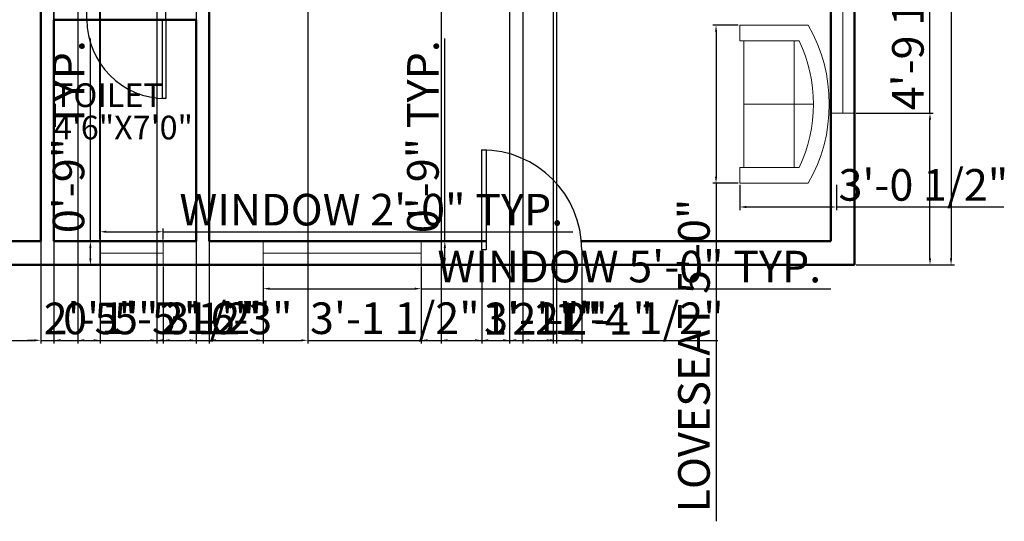
# Model space of a CAD drawing. Units: inches. Extents: x 2744 to 3775, y 2156 to 2963.
# Tile 2 of 4: x 3167 to 3541, y 2156 to 2346. Entities that reach past the tile are written whole.
import ezdxf

# ---------------------------------------------------------------- set-up
doc = ezdxf.new("R2010")
doc.units = ezdxf.units.IN
for name, color, linetype, lineweight in [('A-ANNO-DIMS', 2, 'Continuous', 18), ('A-AREA-IDEN', 7, 'Continuous', 25), ('A-DOOR', 3, 'Continuous', 25), ('A-FURN', 8, 'Continuous', 18), ('A-GLAZ', 4, 'Continuous', 18), ('A-WALL', 7, 'Continuous', 50)]:
    doc.layers.add(name, color=color, linetype=linetype, lineweight=lineweight)
doc.styles.get("Standard").update_dxf_attribs({"font": 'arial.ttf'})
doc.dimstyles.new('ISO-25', dxfattribs={"dimtxt": 12, "dimasz": 2.5, "dimexe": 1.25, "dimexo": 0.625, "dimtad": 1, "dimdec": 1, "dimlunit": 4, "dimtxsty": 'Standard', "dimcen": 2.5, "dimadec": 0, "dimazin": 0, "dimtfac": 1, "dimtdec": 1, "dimtmove": 0, "dimatfit": 3, "dimfxl": 1, "dimarcsym": 0})

# ---------------------------------------------------------------- blocks, each defined once
blk = doc.blocks.new('*U2')
for p, q in [((0, 0), (0, -6)), ((40, 0), (40, -6))]:
    blk.add_line(p, q)
blk.add_lwpolyline([(0, 0), (0, 40), (1.75, 40), (1.75, 0)], close=True)
blk.add_arc((0, 0), 40, 0, 90)
blk = doc.blocks.new('Sofa - Roundback Loveseat 5 ft.')
for p, q in [((0, -32.44198), (0, -5.99998)), ((-24, -33.99998), (-24, -11.46958)), ((-23.9998, -13.38178), (23.99986, -13.38178)), ((24.00004, -33.99998), (24.00004, -11.46958)), ((-24, -32.44198), (24.00004, -32.44198))]:
    blk.add_line(p, q)
for points in [[(-24, -33.99998), (-30, -33.99998), (-30, -7.99998)], [(30.00004, -7.99998), (30.00004, -33.99998), (24.00004, -33.99998)]]:
    blk.add_lwpolyline(points)
for centre, radius, start, end in [((0, -60.24998), 60.24998, 60.13715, 119.8628), ((0, -61.38438), 55.38444, 64.32083, 115.6792)]:
    blk.add_arc(centre, radius, start, end)
blk = doc.blocks.new('*D15')
at = {"layer": 'A-ANNO-DIMS', "color": 0, "lineweight": -2, "transparency": 16777216}
for p, q in [((3484.55, 2757.1), (3521.77, 2757.1)), ((3520.52, 2754.6), (3520.52, 2255.6)), ((3484.55, 2253.1), (3521.77, 2253.1))]:
    blk.add_line(p, q, dxfattribs=at)
at = {"layer": 'A-ANNO-DIMS', "color": 0, "transparency": 16777216}
for points in [[(3520.11, 2754.6), (3520.94, 2754.6), (3520.52, 2757.1)], [(3520.11, 2255.6), (3520.94, 2255.6), (3520.52, 2253.1)]]:
    blk.add_solid(points, dxfattribs=at)
at = {"layer": 'Defpoints', "color": 0, "transparency": 16777216}
for p in [(3483.92, 2757.1), (3483.92, 2253.1), (3520.52, 2253.1)]:
    blk.add_point(p, dxfattribs=at)
at = {"layer": 'A-ANNO-DIMS', "color": 0, "transparency": 16777216, "insert": (3513.88, 2505.1), "char_height": 12, "attachment_point": 5, "rotation": 90}
blk.add_mtext("42'", dxfattribs=at)
blk = doc.blocks.new('WIN-60IN')
blk.add_line((0, 4.5), (60, 4.5))
blk.add_lwpolyline([(0, 9), (60, 9), (60, 0), (0, 0)], close=True)
blk = doc.blocks.new('WIN-24IN')
blk.add_line((0, 4.5), (24, 4.5))
blk.add_lwpolyline([(0, 9), (24, 9), (24, 0), (0, 0)], close=True)
blk = doc.blocks.new('*D18')
at = {"layer": 'A-ANNO-DIMS', "color": 0, "lineweight": -2, "transparency": 16777216}
for p, q in [((3259.32, 2252.48), (3259.32, 2242.85)), ((3319.32, 2252.48), (3319.32, 2242.85)), ((3261.82, 2244.1), (3316.82, 2244.1)), ((3319.32, 2244.1), (3474.92, 2244.1))]:
    blk.add_line(p, q, dxfattribs=at)
at = {"layer": 'A-ANNO-DIMS', "color": 0, "transparency": 16777216}
for points in [[(3261.82, 2244.52), (3261.82, 2243.69), (3259.32, 2244.1)], [(3316.82, 2244.52), (3316.82, 2243.69), (3319.32, 2244.1)]]:
    blk.add_solid(points, dxfattribs=at)
at = {"layer": 'Defpoints', "color": 0, "transparency": 16777216}
for p in [(3259.32, 2253.1), (3319.32, 2253.1), (3319.32, 2244.1)]:
    blk.add_point(p, dxfattribs=at)
at = {"layer": 'A-ANNO-DIMS', "color": 0, "transparency": 16777216, "insert": (3398.37, 2250.94), "char_height": 12, "attachment_point": 5}
blk.add_mtext('WINDOW 5\'-0" TYP.', dxfattribs=at)
blk = doc.blocks.new('*D19')
at = {"layer": 'A-ANNO-DIMS', "color": 0, "lineweight": -2, "transparency": 16777216}
for p, q in [((3328.32, 2262.1), (3328.32, 2339)), ((3319.95, 2262.1), (3329.57, 2262.1)), ((3328.32, 2255.6), (3328.32, 2259.6)), ((3319.95, 2253.1), (3329.57, 2253.1))]:
    blk.add_line(p, q, dxfattribs=at)
at = {"layer": 'A-ANNO-DIMS', "color": 0, "transparency": 16777216}
for points in [[(3327.91, 2259.6), (3328.74, 2259.6), (3328.32, 2262.1)], [(3327.91, 2255.6), (3328.74, 2255.6), (3328.32, 2253.1)]]:
    blk.add_solid(points, dxfattribs=at)
at = {"layer": 'Defpoints', "color": 0, "transparency": 16777216}
for p in [(3319.32, 2262.1), (3328.32, 2262.1), (3319.32, 2253.1)]:
    blk.add_point(p, dxfattribs=at)
at = {"layer": 'A-ANNO-DIMS', "color": 0, "transparency": 16777216, "insert": (3321.57, 2301.8), "char_height": 12, "attachment_point": 5, "rotation": 90}
blk.add_mtext('0\'-9" TYP.', dxfattribs=at)
blk = doc.blocks.new('*D20')
at = {"layer": 'A-ANNO-DIMS', "color": 0, "lineweight": -2, "transparency": 16777216}
for p, q in [((3197.36, 2262.73), (3197.36, 2266.95)), ((3199.86, 2265.7), (3218.86, 2265.7)), ((3221.36, 2262.73), (3221.36, 2266.95)), ((3221.36, 2265.7), (3376.96, 2265.7))]:
    blk.add_line(p, q, dxfattribs=at)
at = {"layer": 'A-ANNO-DIMS', "color": 0, "transparency": 16777216}
for points in [[(3199.86, 2266.12), (3199.86, 2265.29), (3197.36, 2265.7)], [(3218.86, 2266.12), (3218.86, 2265.29), (3221.36, 2265.7)]]:
    blk.add_solid(points, dxfattribs=at)
at = {"layer": 'Defpoints', "color": 0, "transparency": 16777216}
for p in [(3221.36, 2265.7), (3197.36, 2262.1), (3221.36, 2262.1)]:
    blk.add_point(p, dxfattribs=at)
at = {"layer": 'A-ANNO-DIMS', "color": 0, "transparency": 16777216, "insert": (3300.41, 2272.54), "char_height": 12, "attachment_point": 5}
blk.add_mtext('WINDOW 2\'-0" TYP.', dxfattribs=at)
blk = doc.blocks.new('*D21')
at = {"layer": 'A-ANNO-DIMS', "color": 0, "lineweight": -2, "transparency": 16777216}
for p, q in [((3193.76, 2262.1), (3193.76, 2339)), ((3196.74, 2262.1), (3192.51, 2262.1)), ((3193.76, 2255.6), (3193.76, 2259.6)), ((3196.74, 2253.1), (3192.51, 2253.1))]:
    blk.add_line(p, q, dxfattribs=at)
at = {"layer": 'A-ANNO-DIMS', "color": 0, "transparency": 16777216}
for points in [[(3193.35, 2259.6), (3194.18, 2259.6), (3193.76, 2262.1)], [(3193.35, 2255.6), (3194.18, 2255.6), (3193.76, 2253.1)]]:
    blk.add_solid(points, dxfattribs=at)
at = {"layer": 'Defpoints', "color": 0, "transparency": 16777216}
for p in [(3193.76, 2262.1), (3197.36, 2262.1), (3197.36, 2253.1)]:
    blk.add_point(p, dxfattribs=at)
at = {"layer": 'A-ANNO-DIMS', "color": 0, "transparency": 16777216, "insert": (3187.01, 2301.8), "char_height": 12, "attachment_point": 5, "rotation": 90}
blk.add_mtext('0\'-9" TYP.', dxfattribs=at)
blk = doc.blocks.new('*D28')
at = {"layer": 'A-ANNO-DIMS', "color": 0, "lineweight": -2, "transparency": 16777216}
for p, q in [((3439.68, 2344.11), (3430.05, 2344.11)), ((3431.3, 2341.61), (3431.3, 2286.61)), ((3439.68, 2284.11), (3430.05, 2284.11)), ((3431.3, 2284.11), (3431.3, 2155.82))]:
    blk.add_line(p, q, dxfattribs=at)
at = {"layer": 'A-ANNO-DIMS', "color": 0, "transparency": 16777216}
for points in [[(3430.89, 2341.61), (3431.72, 2341.61), (3431.3, 2344.11)], [(3430.89, 2286.61), (3431.72, 2286.61), (3431.3, 2284.11)]]:
    blk.add_solid(points, dxfattribs=at)
at = {"layer": 'Defpoints', "color": 0, "transparency": 16777216}
for p in [(3440.3, 2344.11), (3431.3, 2284.11), (3440.3, 2284.11)]:
    blk.add_point(p, dxfattribs=at)
at = {"layer": 'A-ANNO-DIMS', "color": 0, "transparency": 16777216, "insert": (3424.47, 2218.72), "char_height": 12, "attachment_point": 5, "rotation": 90}
blk.add_mtext('LOVESEAT 5\'-0"', dxfattribs=at)
blk = doc.blocks.new('*D29')
at = {"layer": 'A-ANNO-DIMS', "color": 0, "lineweight": -2, "transparency": 16777216}
for p, q in [((3440.3, 2283.48), (3440.3, 2273.86)), ((3476.97, 2283.48), (3476.97, 2273.86)), ((3442.8, 2275.11), (3474.47, 2275.11)), ((3476.97, 2275.11), (3540.57, 2275.11))]:
    blk.add_line(p, q, dxfattribs=at)
at = {"layer": 'A-ANNO-DIMS', "color": 0, "transparency": 16777216}
for points in [[(3442.8, 2275.52), (3442.8, 2274.69), (3440.3, 2275.11)], [(3474.47, 2275.52), (3474.47, 2274.69), (3476.97, 2275.11)]]:
    blk.add_solid(points, dxfattribs=at)
at = {"layer": 'Defpoints', "color": 0, "transparency": 16777216}
for p in [(3440.3, 2284.11), (3476.97, 2284.11), (3476.97, 2275.11)]:
    blk.add_point(p, dxfattribs=at)
at = {"layer": 'A-ANNO-DIMS', "color": 0, "transparency": 16777216, "insert": (3510.02, 2281.94), "char_height": 12, "attachment_point": 5}
blk.add_mtext('3\'-0 1/2"', dxfattribs=at)
blk = doc.blocks.new('*D34')
at = {"layer": 'A-ANNO-DIMS', "color": 0, "lineweight": -2, "transparency": 16777216}
for p, q in [((3145.86, 2747.48), (3145.86, 2223.25)), ((3174.92, 2747.48), (3174.92, 2223.25)), ((3148.36, 2224.5), (3172.42, 2224.5)), ((3174.92, 2224.5), (3210.78, 2224.5))]:
    blk.add_line(p, q, dxfattribs=at)
at = {"layer": 'A-ANNO-DIMS', "color": 0, "transparency": 16777216}
for points in [[(3148.36, 2224.92), (3148.36, 2224.09), (3145.86, 2224.5)], [(3172.42, 2224.92), (3172.42, 2224.09), (3174.92, 2224.5)]]:
    blk.add_solid(points, dxfattribs=at)
at = {"layer": 'Defpoints', "color": 0, "transparency": 16777216}
for p in [(3145.86, 2748.1), (3174.92, 2748.1), (3174.92, 2224.5)]:
    blk.add_point(p, dxfattribs=at)
at = {"layer": 'A-ANNO-DIMS', "color": 0, "transparency": 16777216, "insert": (3194.1, 2231.26), "char_height": 12, "attachment_point": 5}
blk.add_mtext('2\'-5"', dxfattribs=at)
blk = doc.blocks.new('*D35')
at = {"layer": 'A-ANNO-DIMS', "color": 0, "lineweight": -2, "transparency": 16777216}
for p, q in [((3179.92, 2747.48), (3179.92, 2223.25)), ((3197.52, 2747.48), (3197.52, 2223.25)), ((3182.42, 2224.5), (3195.02, 2224.5)), ((3197.52, 2224.5), (3260.01, 2224.5))]:
    blk.add_line(p, q, dxfattribs=at)
at = {"layer": 'A-ANNO-DIMS', "color": 0, "transparency": 16777216}
for points in [[(3182.42, 2224.92), (3182.42, 2224.09), (3179.92, 2224.5)], [(3195.02, 2224.92), (3195.02, 2224.09), (3197.52, 2224.5)]]:
    blk.add_solid(points, dxfattribs=at)
at = {"layer": 'Defpoints', "color": 0, "transparency": 16777216}
for p in [(3179.92, 2748.1), (3197.52, 2748.1), (3197.52, 2224.5)]:
    blk.add_point(p, dxfattribs=at)
at = {"layer": 'A-ANNO-DIMS', "color": 0, "transparency": 16777216, "insert": (3230.02, 2231.33), "char_height": 12, "attachment_point": 5}
blk.add_mtext('1\'-5 1/2"', dxfattribs=at)
blk = doc.blocks.new('*D36')
at = {"layer": 'A-ANNO-DIMS', "color": 0, "lineweight": -2, "transparency": 16777216}
for p, q in [((3326.88, 2747.48), (3326.88, 2223.25)), ((3352.92, 2747.48), (3352.92, 2223.25)), ((3329.38, 2224.5), (3350.42, 2224.5)), ((3352.92, 2224.5), (3388.78, 2224.5))]:
    blk.add_line(p, q, dxfattribs=at)
at = {"layer": 'A-ANNO-DIMS', "color": 0, "transparency": 16777216}
for points in [[(3329.38, 2224.92), (3329.38, 2224.09), (3326.88, 2224.5)], [(3350.42, 2224.92), (3350.42, 2224.09), (3352.92, 2224.5)]]:
    blk.add_solid(points, dxfattribs=at)
at = {"layer": 'Defpoints', "color": 0, "transparency": 16777216}
for p in [(3326.88, 2748.1), (3352.92, 2748.1), (3352.92, 2224.5)]:
    blk.add_point(p, dxfattribs=at)
at = {"layer": 'A-ANNO-DIMS', "color": 0, "transparency": 16777216, "insert": (3372.1, 2231.15), "char_height": 12, "attachment_point": 5}
blk.add_mtext('2\'-2"', dxfattribs=at)
blk = doc.blocks.new('*D37')
at = {"layer": 'A-ANNO-DIMS', "color": 0, "lineweight": -2, "transparency": 16777216}
for p, q in [((3357.92, 2747.48), (3357.92, 2223.25)), ((3370.78, 2747.48), (3370.78, 2223.25)), ((3360.42, 2224.5), (3368.28, 2224.5)), ((3370.78, 2224.5), (3405.3, 2224.5))]:
    blk.add_line(p, q, dxfattribs=at)
at = {"layer": 'A-ANNO-DIMS', "color": 0, "transparency": 16777216}
for points in [[(3360.42, 2224.92), (3360.42, 2224.09), (3357.92, 2224.5)], [(3368.28, 2224.92), (3368.28, 2224.09), (3370.78, 2224.5)]]:
    blk.add_solid(points, dxfattribs=at)
at = {"layer": 'Defpoints', "color": 0, "transparency": 16777216}
for p in [(3357.92, 2748.1), (3370.78, 2748.1), (3370.78, 2224.5)]:
    blk.add_point(p, dxfattribs=at)
at = {"layer": 'A-ANNO-DIMS', "color": 0, "transparency": 16777216, "insert": (3389.29, 2231.15), "char_height": 12, "attachment_point": 5}
blk.add_mtext('1\'-1"', dxfattribs=at)
blk = doc.blocks.new('*D39')
at = {"layer": 'A-ANNO-DIMS', "color": 0, "lineweight": -2, "transparency": 16777216}
for p, q in [((3179.92, 2262.73), (3179.92, 2786.95)), ((3182.42, 2785.7), (3194.86, 2785.7)), ((3197.36, 2262.73), (3197.36, 2786.95)), ((3197.36, 2785.7), (3259.85, 2785.7))]:
    blk.add_line(p, q, dxfattribs=at)
at = {"layer": 'A-ANNO-DIMS', "color": 0, "transparency": 16777216}
for points in [[(3182.42, 2786.12), (3182.42, 2785.29), (3179.92, 2785.7)], [(3194.86, 2786.12), (3194.86, 2785.29), (3197.36, 2785.7)]]:
    blk.add_solid(points, dxfattribs=at)
at = {"layer": 'Defpoints', "color": 0, "transparency": 16777216}
for p in [(3197.36, 2785.7), (3179.92, 2262.1), (3197.36, 2262.1)]:
    blk.add_point(p, dxfattribs=at)
at = {"layer": 'A-ANNO-DIMS', "color": 0, "transparency": 16777216, "insert": (3229.85, 2792.53), "char_height": 12, "attachment_point": 5}
blk.add_mtext('1\'-5 1/2"', dxfattribs=at)
blk = doc.blocks.new('*D40')
at = {"layer": 'A-ANNO-DIMS', "color": 0, "lineweight": -2, "transparency": 16777216}
for p, q in [((3221.36, 2252.48), (3221.36, 2223.25)), ((3259.32, 2252.48), (3259.32, 2223.25)), ((3223.86, 2224.5), (3256.82, 2224.5))]:
    blk.add_line(p, q, dxfattribs=at)
at = {"layer": 'A-ANNO-DIMS', "color": 0, "transparency": 16777216}
for points in [[(3223.86, 2224.92), (3223.86, 2224.09), (3221.36, 2224.5)], [(3256.82, 2224.92), (3256.82, 2224.09), (3259.32, 2224.5)]]:
    blk.add_solid(points, dxfattribs=at)
at = {"layer": 'Defpoints', "color": 0, "transparency": 16777216}
for p in [(3221.36, 2253.1), (3259.32, 2253.1), (3259.32, 2224.5)]:
    blk.add_point(p, dxfattribs=at)
at = {"layer": 'A-ANNO-DIMS', "color": 0, "transparency": 16777216, "insert": (3240.34, 2231.26), "char_height": 12, "attachment_point": 5}
blk.add_mtext('3\'-2"', dxfattribs=at)
blk = doc.blocks.new('*D41')
at = {"layer": 'A-ANNO-DIMS', "color": 0, "lineweight": -2, "transparency": 16777216}
for p, q in [((3319.32, 2252.48), (3319.32, 2223.25)), ((3342.33, 2252.48), (3342.33, 2223.25)), ((3321.82, 2224.5), (3339.83, 2224.5)), ((3342.33, 2224.5), (3386.18, 2224.5))]:
    blk.add_line(p, q, dxfattribs=at)
at = {"layer": 'A-ANNO-DIMS', "color": 0, "transparency": 16777216}
for points in [[(3321.82, 2224.92), (3321.82, 2224.09), (3319.32, 2224.5)], [(3339.83, 2224.92), (3339.83, 2224.09), (3342.33, 2224.5)]]:
    blk.add_solid(points, dxfattribs=at)
at = {"layer": 'Defpoints', "color": 0, "transparency": 16777216}
for p in [(3319.32, 2253.1), (3342.33, 2253.1), (3342.33, 2224.5)]:
    blk.add_point(p, dxfattribs=at)
at = {"layer": 'A-ANNO-DIMS', "color": 0, "transparency": 16777216, "insert": (3365.5, 2231.15), "char_height": 12, "attachment_point": 5}
blk.add_mtext('1\'-11"', dxfattribs=at)
blk = doc.blocks.new('*D42')
at = {"layer": 'A-ANNO-DIMS', "color": 0, "lineweight": -2, "transparency": 16777216}
for p, q in [((3342.33, 2252.48), (3342.33, 2223.25)), ((3380.33, 2252.48), (3380.33, 2223.25)), ((3344.83, 2224.5), (3377.83, 2224.5))]:
    blk.add_line(p, q, dxfattribs=at)
at = {"layer": 'A-ANNO-DIMS', "color": 0, "transparency": 16777216}
for points in [[(3344.83, 2224.92), (3344.83, 2224.09), (3342.33, 2224.5)], [(3377.83, 2224.92), (3377.83, 2224.09), (3380.33, 2224.5)]]:
    blk.add_solid(points, dxfattribs=at)
at = {"layer": 'Defpoints', "color": 0, "transparency": 16777216}
for p in [(3342.33, 2253.1), (3380.33, 2253.1), (3380.33, 2224.5)]:
    blk.add_point(p, dxfattribs=at)
at = {"layer": 'A-ANNO-DIMS', "color": 0, "transparency": 16777216, "insert": (3361.33, 2231.26), "char_height": 12, "attachment_point": 5}
blk.add_mtext('3\'-2"', dxfattribs=at)
blk = doc.blocks.new('*D43')
at = {"layer": 'A-ANNO-DIMS', "color": 0, "lineweight": -2, "transparency": 16777216}
for p, q in [((3512.52, 2310.69), (3512.52, 2374.78)), ((3484.55, 2310.69), (3513.77, 2310.69)), ((3512.52, 2255.6), (3512.52, 2308.19)), ((3484.55, 2253.1), (3513.77, 2253.1))]:
    blk.add_line(p, q, dxfattribs=at)
at = {"layer": 'A-ANNO-DIMS', "color": 0, "transparency": 16777216}
for points in [[(3512.11, 2308.19), (3512.94, 2308.19), (3512.52, 2310.69)], [(3512.11, 2255.6), (3512.94, 2255.6), (3512.52, 2253.1)]]:
    blk.add_solid(points, dxfattribs=at)
at = {"layer": 'Defpoints', "color": 0, "transparency": 16777216}
for p in [(3483.92, 2310.69), (3512.52, 2310.69), (3483.92, 2253.1)]:
    blk.add_point(p, dxfattribs=at)
at = {"layer": 'A-ANNO-DIMS', "color": 0, "transparency": 16777216, "insert": (3505.69, 2343.99), "char_height": 12, "attachment_point": 5, "rotation": 90}
blk.add_mtext('4\'-9 1/2"', dxfattribs=at)
blk = doc.blocks.new('*D45')
at = {"layer": 'A-ANNO-DIMS', "color": 0, "lineweight": -2, "transparency": 16777216}
for p, q in [((3188.98, 2574.48), (3188.98, 2223.25)), ((3218.98, 2574.48), (3218.98, 2223.25)), ((3191.48, 2224.5), (3216.48, 2224.5)), ((3218.98, 2224.5), (3254.83, 2224.5))]:
    blk.add_line(p, q, dxfattribs=at)
at = {"layer": 'A-ANNO-DIMS', "color": 0, "transparency": 16777216}
for points in [[(3191.48, 2224.92), (3191.48, 2224.09), (3188.98, 2224.5)], [(3216.48, 2224.92), (3216.48, 2224.09), (3218.98, 2224.5)]]:
    blk.add_solid(points, dxfattribs=at)
at = {"layer": 'Defpoints', "color": 0, "transparency": 16777216}
for p in [(3188.98, 2575.1), (3218.98, 2575.1), (3218.98, 2224.5)]:
    blk.add_point(p, dxfattribs=at)
at = {"layer": 'A-ANNO-DIMS', "color": 0, "transparency": 16777216, "insert": (3238.16, 2231.26), "char_height": 12, "attachment_point": 5}
blk.add_mtext('2\'-6"', dxfattribs=at)
blk = doc.blocks.new('*D46')
at = {"layer": 'A-ANNO-DIMS', "color": 0, "lineweight": -2, "transparency": 16777216}
for p, q in [((3218.97, 2579.48), (3218.97, 2223.25)), ((3233.92, 2579.48), (3233.92, 2223.25)), ((3221.47, 2224.5), (3231.42, 2224.5)), ((3233.92, 2224.5), (3268.44, 2224.5))]:
    blk.add_line(p, q, dxfattribs=at)
at = {"layer": 'A-ANNO-DIMS', "color": 0, "transparency": 16777216}
for points in [[(3221.47, 2224.92), (3221.47, 2224.09), (3218.97, 2224.5)], [(3231.42, 2224.92), (3231.42, 2224.09), (3233.92, 2224.5)]]:
    blk.add_solid(points, dxfattribs=at)
at = {"layer": 'Defpoints', "color": 0, "transparency": 16777216}
for p in [(3218.97, 2580.1), (3233.92, 2580.1), (3233.92, 2224.5)]:
    blk.add_point(p, dxfattribs=at)
at = {"layer": 'A-ANNO-DIMS', "color": 0, "transparency": 16777216, "insert": (3252.43, 2231.26), "char_height": 12, "attachment_point": 5}
blk.add_mtext('1\'-3"', dxfattribs=at)
blk = doc.blocks.new('*D47')
at = {"layer": 'A-ANNO-DIMS', "color": 0, "lineweight": -2, "transparency": 16777216}
for p, q in [((3238.92, 2579.48), (3238.92, 2223.25)), ((3276.3, 2578.98), (3276.3, 2223.25)), ((3241.42, 2224.5), (3273.8, 2224.5)), ((3276.3, 2224.5), (3339.9, 2224.5))]:
    blk.add_line(p, q, dxfattribs=at)
at = {"layer": 'A-ANNO-DIMS', "color": 0, "transparency": 16777216}
for points in [[(3241.42, 2224.92), (3241.42, 2224.09), (3238.92, 2224.5)], [(3273.8, 2224.92), (3273.8, 2224.09), (3276.3, 2224.5)]]:
    blk.add_solid(points, dxfattribs=at)
at = {"layer": 'Defpoints', "color": 0, "transparency": 16777216}
for p in [(3238.92, 2580.1), (3276.3, 2579.6), (3276.3, 2224.5)]:
    blk.add_point(p, dxfattribs=at)
at = {"layer": 'A-ANNO-DIMS', "color": 0, "transparency": 16777216, "insert": (3309.35, 2231.34), "char_height": 12, "attachment_point": 5}
blk.add_mtext('3\'-1 1/2"', dxfattribs=at)
blk = doc.blocks.new('*D59')
at = {"layer": 'A-ANNO-DIMS', "color": 0, "lineweight": -2, "transparency": 16777216}
for p, q in [((3174.92, 2350.48), (3174.92, 2223.25)), ((3179.92, 2345.48), (3179.92, 2223.25)), ((3172.42, 2224.5), (3169.92, 2224.5)), ((3174.92, 2224.5), (3179.92, 2224.5)), ((3182.42, 2224.5), (3218.07, 2224.5))]:
    blk.add_line(p, q, dxfattribs=at)
at = {"layer": 'A-ANNO-DIMS', "color": 0, "transparency": 16777216}
for points in [[(3172.42, 2224.92), (3172.42, 2224.09), (3174.92, 2224.5)], [(3182.42, 2224.92), (3182.42, 2224.09), (3179.92, 2224.5)]]:
    blk.add_solid(points, dxfattribs=at)
at = {"layer": 'Defpoints', "color": 0, "transparency": 16777216}
for p in [(3174.92, 2351.1), (3179.92, 2346.1), (3179.92, 2224.5)]:
    blk.add_point(p, dxfattribs=at)
at = {"layer": 'A-ANNO-DIMS', "color": 0, "transparency": 16777216, "insert": (3201.5, 2231.26), "char_height": 12, "attachment_point": 5}
blk.add_mtext('0\'-5"', dxfattribs=at)
blk = doc.blocks.new('*D65')
at = {"layer": 'A-ANNO-DIMS', "color": 0, "lineweight": -2, "transparency": 16777216}
for p, q in [((3352.92, 2658.48), (3352.92, 2223.25)), ((3369.47, 2658.48), (3369.47, 2223.25)), ((3355.42, 2224.5), (3366.97, 2224.5)), ((3369.47, 2224.5), (3431.96, 2224.5))]:
    blk.add_line(p, q, dxfattribs=at)
at = {"layer": 'A-ANNO-DIMS', "color": 0, "transparency": 16777216}
for points in [[(3355.42, 2224.92), (3355.42, 2224.09), (3352.92, 2224.5)], [(3366.97, 2224.92), (3366.97, 2224.09), (3369.47, 2224.5)]]:
    blk.add_solid(points, dxfattribs=at)
at = {"layer": 'Defpoints', "color": 0, "transparency": 16777216}
for p in [(3352.92, 2659.1), (3369.47, 2659.1), (3369.47, 2224.5)]:
    blk.add_point(p, dxfattribs=at)
at = {"layer": 'A-ANNO-DIMS', "color": 0, "transparency": 16777216, "insert": (3401.97, 2231.33), "char_height": 12, "attachment_point": 5}
blk.add_mtext('1\'-4 1/2"', dxfattribs=at)

msp = doc.modelspace()

# ---------------------------------------------------------------- linework, layer by layer
at = {"layer": 'A-WALL'}
for p, q in [((3483.92, 2757.1), (3483.92, 2253.1)), ((3238.92, 2262.1), (3238.92, 2435.1)), ((3474.92, 2430.1), (3474.92, 2262.1)), ((3174.92, 2262.1), (3174.92, 2351.1)), ((3179.92, 2262.1), (3179.92, 2346.1)), ((3233.92, 2346.1), (3179.92, 2346.1)), ((3233.92, 2262.1), (3233.92, 2346.1)), ((3174.92, 2262.1), (3065.92, 2262.1)), ((3233.92, 2262.1), (3179.92, 2262.1)), ((3344, 2262.1), (3238.92, 2262.1)), ((3474.92, 2262.1), (3380.19, 2262.1)), ((3483.92, 2253.1), (3003.92, 2253.1))]:
    msp.add_line(p, q, dxfattribs=at)

# ---------------------------------------------------------------- block references
at = {"layer": 'A-DOOR', "xscale": 0.75, "yscale": 0.75, "zscale": 0.75, "rotation": 180}
msp.add_blockref('*U2', (3222.43, 2346.25), dxfattribs=at)
at = {"layer": 'A-DOOR', "xscale": 0.95, "yscale": 0.95, "zscale": 0.95}
msp.add_blockref('*U2', (3342.33, 2258.8), dxfattribs=at)
at = {"layer": 'A-FURN', "rotation": 270}
msp.add_blockref('Sofa - Roundback Loveseat 5 ft.', (3474.3, 2314.11), dxfattribs=at)
at = {"layer": 'A-GLAZ', "rotation": 270.0000000000006}
msp.add_blockref('WIN-60IN', (3474.92, 2370.69), dxfattribs=at)
at = {"layer": 'A-GLAZ'}
for name, p in [('WIN-24IN', (3197.36, 2253.1)), ('WIN-60IN', (3259.32, 2253.1))]:
    msp.add_blockref(name, p, dxfattribs=at)

# ---------------------------------------------------------------- texts
at = {"layer": 'A-AREA-IDEN'}
for s, p in [('TOILET', (3179.92, 2313.04)), ('4\'6"X7\'0"', (3179.92, 2300.75))]:
    msp.add_text(s, height=9, dxfattribs=at).set_placement(p)

# ---------------------------------------------------------------- dimensions: what is measured, and where the dimension line sits
at = {"layer": 'A-ANNO-DIMS'}
for base, p1, p2, picture, middle in [((3197.36, 2785.7), (3179.92, 2262.1), (3197.36, 2262.1), '*D39', (3229.85, 2792.53)), ((3174.92, 2224.5), (3145.86, 2748.1), (3174.92, 2748.1), '*D34', (3194.1, 2231.26)), ((3197.52, 2224.5), (3179.92, 2748.1), (3197.52, 2748.1), '*D35', (3230.02, 2231.33)), ((3352.92, 2224.5), (3326.88, 2748.1), (3352.92, 2748.1), '*D36', (3372.1, 2231.15)), ((3370.78, 2224.5), (3357.92, 2748.1), (3370.78, 2748.1), '*D37', (3389.29, 2231.15)), ((3369.4749, 2224.505), (3352.9224, 2659.105), (3369.4749, 2659.105), '*D65', (3401.9655, 2231.3346)), ((3233.9224, 2224.505), (3218.9746, 2580.105), (3233.9224, 2580.105), '*D46', (3252.4322, 2231.2609)), ((3276.3, 2224.5), (3238.92, 2580.1), (3276.3, 2579.6), '*D47', (3309.35, 2231.34)), ((3218.98, 2224.5), (3188.98, 2575.1), (3218.98, 2575.1), '*D45', (3238.16, 2231.26)), ((3179.92, 2224.5), (3174.92, 2351.1), (3179.92, 2346.1), '*D59', (3201.5, 2231.26)), ((3476.97, 2275.11), (3440.3, 2284.11), (3476.97, 2284.11), '*D29', (3510.02, 2281.94)), ((3259.32, 2224.5), (3221.36, 2253.1), (3259.32, 2253.1), '*D40', (3240.34, 2231.26)), ((3342.33, 2224.5), (3319.32, 2253.1), (3342.33, 2253.1), '*D41', (3365.5, 2231.15)), ((3380.33, 2224.5), (3342.33, 2253.1), (3380.33, 2253.1), '*D42', (3361.33, 2231.26))]:
    dim = msp.add_linear_dim(base=base, p1=p1, p2=p2, dimstyle='ISO-25', override={"dimdec": 1, "dimlfac": 1, "dimrnd": 0, "dimzin": 1, "dimdsep": 46, "dimlunit": 4, "dimfrac": 2}, dxfattribs=at)
    dim.commit()
    dim.dimension.update_dxf_attribs({"geometry": picture, "text_midpoint": middle})
for base, p1, p2, override, picture, middle in [((3520.52, 2253.1), (3483.92, 2757.1), (3483.92, 2253.1), {"dimclrd": 0, "dimclre": 0, "dimclrt": 0}, '*D15', (3513.88, 2505.1)), ((3512.52, 2310.69), (3483.92, 2253.1), (3483.92, 2310.69), {"dimdec": 1, "dimlfac": 1, "dimrnd": 0, "dimzin": 1, "dimdsep": 46, "dimlunit": 4, "dimfrac": 2}, '*D43', (3505.69, 2343.99))]:
    dim = msp.add_linear_dim(base=base, p1=p1, p2=p2, angle=90, dimstyle='ISO-25', override=override, dxfattribs=at)
    dim.commit()
    dim.dimension.update_dxf_attribs({"geometry": picture, "text_midpoint": middle})
for base, p1, p2, angle, text, picture, middle in [((3431.3, 2284.11), (3440.3, 2344.11), (3440.3, 2284.11), 270, 'LOVESEAT <>', '*D28', (3424.47, 2218.72)), ((3193.76, 2262.1), (3197.36, 2253.1), (3197.36, 2262.1), 90, '<> TYP.', '*D21', (3187.01, 2301.8)), ((3328.32, 2262.1), (3319.32, 2253.1), (3319.32, 2262.1), 90, '<> TYP.', '*D19', (3321.57, 2301.8))]:
    dim = msp.add_linear_dim(base=base, p1=p1, p2=p2, angle=angle, text=text, dimstyle='ISO-25', override={"dimdec": 1, "dimlfac": 1, "dimrnd": 0, "dimzin": 1, "dimdsep": 46, "dimlunit": 4, "dimfrac": 2}, dxfattribs=at)
    dim.commit()
    dim.dimension.update_dxf_attribs({"geometry": picture, "text_midpoint": middle})
for base, p1, p2, picture, middle in [((3221.36, 2265.7), (3197.36, 2262.1), (3221.36, 2262.1), '*D20', (3300.41, 2272.54)), ((3319.32, 2244.1), (3259.32, 2253.1), (3319.32, 2253.1), '*D18', (3398.37, 2250.94))]:
    dim = msp.add_linear_dim(base=base, p1=p1, p2=p2, text='WINDOW <> TYP.', dimstyle='ISO-25', override={"dimdec": 1, "dimlfac": 1, "dimrnd": 0, "dimzin": 1, "dimdsep": 46, "dimlunit": 4, "dimfrac": 2}, dxfattribs=at)
    dim.commit()
    dim.dimension.update_dxf_attribs({"geometry": picture, "text_midpoint": middle})

doc.saveas('drawing.dxf')
